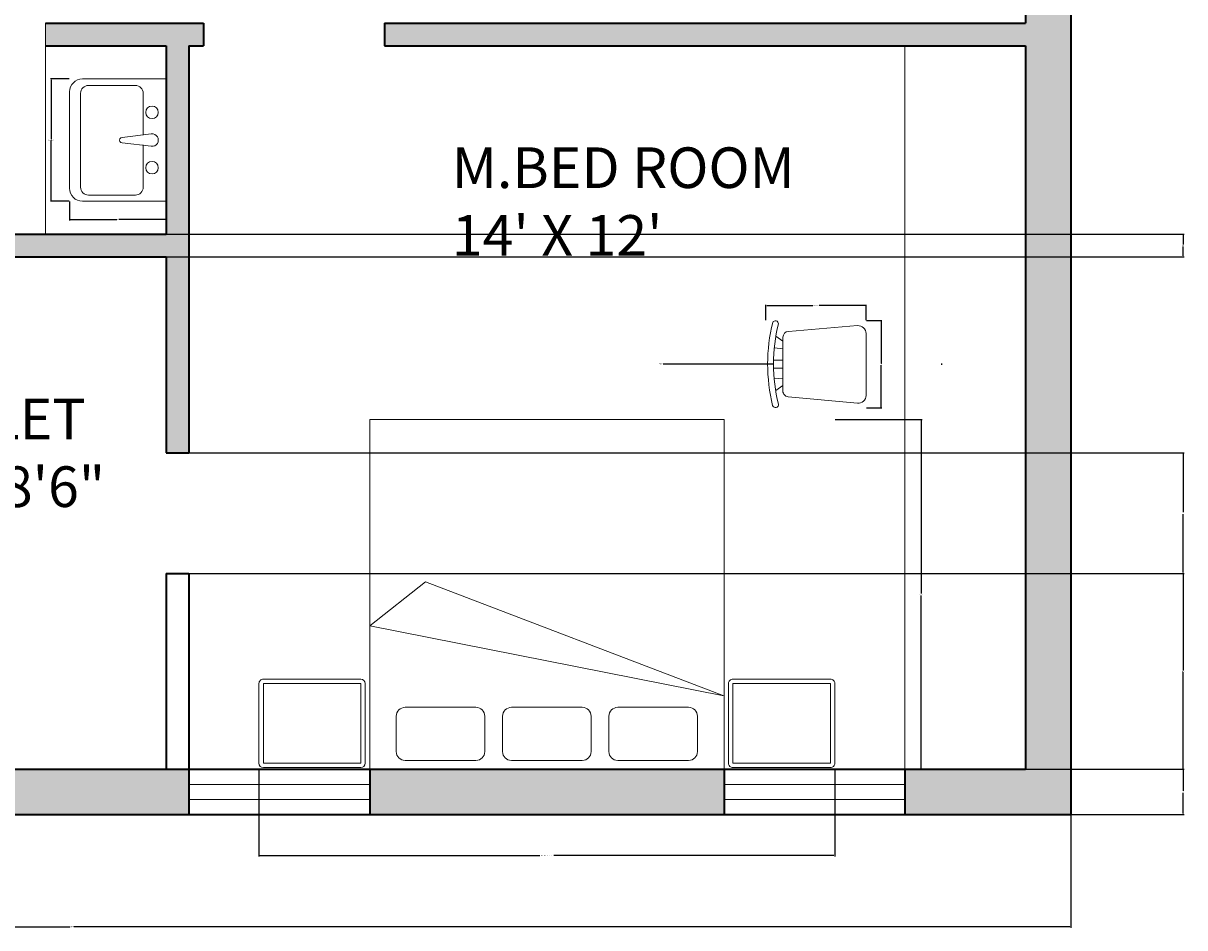
# Model space of a CAD drawing. Units: inches. Extents: x 2 to 2806, y 1095 to 1587.
# Tile 2 of 4: x 2575 to 2806, y 1095 to 1275. Entities that reach past the tile are written whole.
import ezdxf

# ---------------------------------------------------------------- set-up
doc = ezdxf.new("R2010")
doc.units = ezdxf.units.IN
for name, color, linetype, lineweight in [('A-ANNO-DIMS', 2, 'Continuous', 18), ('A-AREA-IDEN', 7, 'Continuous', 25), ('A-FLOR-CASE', 34, 'Continuous', 18), ('A-FLOR-FIXT', 9, 'Continuous', 18), ('A-FURN', 8, 'Continuous', 18), ('A-GLAZ', 4, 'Continuous', 18), ('A-WALL', 7, 'Continuous', 35)]:
    doc.layers.add(name, color=color, linetype=linetype, lineweight=lineweight)
doc.layers.add('A-WALL-PATT', color=18, linetype='Continuous', lineweight=13, true_color=0x000000)
doc.styles.get("Standard").update_dxf_attribs({"font": 'arial.ttf'})
doc.dimstyles.get("Standard").update_dxf_attribs({"dimtxt": 0.18, "dimasz": 0.18, "dimexe": 0.18, "dimexo": 0.0625, "dimgap": 0.09, "dimtad": 0, "dimtih": 1, "dimtoh": 1, "dimdec": 4, "dimzin": 0, "dimdsep": 46, "dimtxsty": 'Standard', "dimcen": 0.09, "dimadec": 0, "dimazin": 0, "dimtfac": 1, "dimtdec": 4, "dimtofl": 0, "dimtmove": 0, "dimatfit": 3, "dimfxl": 1, "dimtolj": 1, "dimtzin": 0, "dimarcsym": 0})

# ---------------------------------------------------------------- blocks, each defined once
blk = doc.blocks.new('A$C34D52403')
for p, q in [((0, 0.4572), (0, 0.061)), ((0.5791, 0.4572), (0, 0.4572)), ((0.5791, 0.061), (0.5791, 0.4572)), ((0.277, 0.2492), (0.2602, 0.387)), ((0.3022, 0.2492), (0.319, 0.387)), ((0.2663, 0.3489), (0.0679, 0.3489)), ((0.5131, 0.3489), (0.3128, 0.3489)), ((0.0308, 0.3118), (0.0308, 0.0892)), ((0.5502, 0.0892), (0.5502, 0.3118)), ((0.0679, 0.0521), (0.5131, 0.0521)), ((0.061, 0), (0.5182, 0))]:
    blk.add_line(p, q)
for centre in [(0.1584, 0.3906), (0.4208, 0.3906)]:
    blk.add_circle(centre, 0.0296)
for centre, radius, start, end in [((0.2896, 0.3906), 0.0296, 353.0422, 186.9578), ((0.0679, 0.3118), 0.0371, 90, 180), ((0.5131, 0.3118), 0.0371, 0, 90), ((0.2896, 0.2491), 0.0125, 179.3528, 0.6472), ((0.061, 0.061), 0.061, 180, 270), ((0.0679, 0.0892), 0.0371, 180, 270), ((0.5131, 0.0892), 0.0371, 270, 0), ((0.5182, 0.061), 0.061, 270, 0)]:
    blk.add_arc(centre, radius, start, end)
blk = doc.blocks.new('A$C793B20D3')
for p, q in [((0.625, 0), (0.625, 1.975)), ((2.625, 1.975), (0.625, 1.975)), ((2.625, 0), (2.625, 1.975)), ((0.575, 1.9405), (0.025, 1.9405)), ((0.025, 1.9405), (0.025, 1.4905)), ((0.575, 1.4905), (0.575, 1.9405)), ((0.825, 1.925), (1.225, 1.925)), ((1.425, 1.925), (1.825, 1.925)), ((2.025, 1.925), (2.425, 1.925)), ((2.65, 1.4905), (2.65, 1.9405)), ((2.675, 1.9655), (3.225, 1.9655)), ((3.25, 1.9405), (3.25, 1.4905)), ((0.775, 1.675), (0.775, 1.875)), ((1.275, 1.675), (1.275, 1.875)), ((1.375, 1.675), (1.375, 1.875)), ((1.875, 1.675), (1.875, 1.875)), ((1.975, 1.675), (1.975, 1.875)), ((2.475, 1.675), (2.475, 1.875)), ((0.825, 1.625), (1.225, 1.625)), ((1.425, 1.625), (1.825, 1.625)), ((2.025, 1.625), (2.425, 1.625)), ((0.6256, 1.5604), (2.3107, 0.9169)), ((0.6256, 1.5604), (2.625, 1.1646)), ((0.025, 1.4905), (0.575, 1.4905)), ((3.225, 1.4655), (2.675, 1.4655)), ((2.3107, 0.9169), (2.625, 1.1646)), ((2.625, 0), (0.625, 0))]:
    blk.add_line(p, q)
at = {"flags": 128}
blk.add_lwpolyline([(0, 1.9405), (0, 1.4905, 0.414214), (0.025, 1.4655), (0.575, 1.4655, 0.414214), (0.6, 1.4905), (0.6, 1.9405, 0.414214), (0.575, 1.9655), (0.025, 1.9655, 0.414214)], format="xyb", close=True, dxfattribs=at)
blk.add_lwpolyline([(3.225, 1.9405), (3.225, 1.4905), (2.675, 1.4905), (2.675, 1.9405)], close=True)
for centre, radius, start, end in [((0.825, 1.875), 0.05, 90, 180), ((1.225, 1.875), 0.05, 0, 90), ((1.425, 1.875), 0.05, 90, 180), ((1.825, 1.875), 0.05, 0, 90), ((2.025, 1.875), 0.05, 90, 180), ((2.425, 1.875), 0.05, 0, 90), ((2.675, 1.9405), 0.025, 90, 180), ((3.225, 1.9405), 0.025, 0, 90), ((0.825, 1.675), 0.05, 180, 270), ((1.225, 1.675), 0.05, 270, 0), ((1.425, 1.675), 0.05, 180, 270), ((1.825, 1.675), 0.05, 270, 0), ((2.025, 1.675), 0.05, 180, 270), ((2.425, 1.675), 0.05, 270, 0), ((2.675, 1.4905), 0.025, 180, 270), ((3.225, 1.4905), 0.025, 270, 0)]:
    blk.add_arc(centre, radius, start, end)
blk = doc.blocks.new('A$C309F5002')
for p, q in [((111.5, 420, 1920), (85.9, 456.6, 1920)), ((355.3, 420, 1920), (91.6, 420, 1920)), ((149.5, 420, 1920), (144.7, 463.9, 1920)), ((199.7, 420, 1920), (199.7, 467, 1920)), ((239.7, 420, 1920), (239.7, 467, 1920)), ((297.4, 420, 1920), (302.1, 463.3, 1920)), ((335.4, 420, 1920), (360.3, 455.6, 1920)), ((54.2, 392.8, 1920), (21.8, 43.7, 1920)), ((414.1, 43.3, 1920), (385.2, 392.5, 1920)), ((61.6, 0, 1920), (374.3, 0, 1920))]:
    blk.add_line(p, q)
for centre, radius, start, end in [((14.6, 457.4, 1920), 15, 105.30285, 282.25466), ((220.1, -382.5, 1920), 879.7, 76.18316, 103.77876), ((423.1, 458.1, 1920), 15.4, 269.91655, 62.44977), ((220.1, -382.5, 1920), 849.7, 76.18316, 103.77876), ((85.3, 389.4, 1920), 31.2, 78.31932, 173.81515), ((355.3, 390, 1920), 30, 4.74462, 90), ((61.6, 40, 1920), 40, 174.69095, 270), ((374.3, 40, 1920), 40, 270, 4.74462)]:
    blk.add_arc(centre, radius, start, end)
blk = doc.blocks.new('WIN-GLAZ-36x9')
for p, q in [((0, 3), (36, 3)), ((0, 0), (36, 0))]:
    blk.add_line(p, q)
blk = doc.blocks.new('*D30')
at = {"layer": 'A-ANNO-DIMS', "color": 0, "lineweight": -2, "transparency": 16777216}
for p, q in [((2621.61, 1126.15), (2621.61, 1108.85)), ((2736.17, 1126.15), (2736.17, 1108.85)), ((2621.79, 1109.03), (2677.51, 1109.03)), ((2735.99, 1109.03), (2680.28, 1109.03))]:
    blk.add_line(p, q, dxfattribs=at)
at = {"layer": 'A-ANNO-DIMS', "color": 0, "transparency": 16777216}
for points in [[(2621.79, 1109.06), (2621.79, 1109), (2621.61, 1109.03)], [(2735.99, 1109.06), (2735.99, 1109), (2736.17, 1109.03)]]:
    blk.add_solid(points, dxfattribs=at)
at = {"layer": 'Defpoints', "color": 0, "transparency": 16777216}
for p in [(2621.61, 1126.21), (2736.17, 1126.21), (2621.61, 1109.03)]:
    blk.add_point(p, dxfattribs=at)
at = {"layer": 'A-ANNO-DIMS', "color": 0, "transparency": 16777216, "insert": (2678.89, 1109.03), "char_height": 0.18, "attachment_point": 5}
blk.add_mtext('\\A1;BED GROUP 115 TYP.', dxfattribs=at)
blk = doc.blocks.new('*D31')
at = {"layer": 'A-ANNO-DIMS', "color": 0, "lineweight": -2, "transparency": 16777216}
for p, q in [((2736.24, 1195.83), (2753.54, 1195.83)), ((2753.36, 1195.65), (2753.36, 1161.2)), ((2753.36, 1126.39), (2753.36, 1160.84)), ((2736.24, 1126.21), (2753.54, 1126.21))]:
    blk.add_line(p, q, dxfattribs=at)
at = {"layer": 'A-ANNO-DIMS', "color": 0, "transparency": 16777216}
for points in [[(2753.33, 1195.65), (2753.39, 1195.65), (2753.36, 1195.83)], [(2753.33, 1126.39), (2753.39, 1126.39), (2753.36, 1126.21)]]:
    blk.add_solid(points, dxfattribs=at)
at = {"layer": 'Defpoints', "color": 0, "transparency": 16777216}
for p in [(2736.17, 1195.83), (2736.17, 1126.21), (2753.36, 1126.21)]:
    blk.add_point(p, dxfattribs=at)
at = {"layer": 'A-ANNO-DIMS', "color": 0, "transparency": 16777216, "insert": (2753.36, 1161.02), "char_height": 0.18, "attachment_point": 5}
blk.add_mtext('\\A1;70 TYP.', dxfattribs=at)
blk = doc.blocks.new('*D46')
at = {"layer": 'A-ANNO-DIMS', "color": 0, "lineweight": -2, "transparency": 16777216}
for p, q in [((2583.87, 1263.63), (2580.11, 1263.63)), ((2580.29, 1263.45), (2580.29, 1251.65)), ((2580.29, 1239.48), (2580.29, 1251.28)), ((2583.87, 1239.3), (2580.11, 1239.3))]:
    blk.add_line(p, q, dxfattribs=at)
at = {"layer": 'A-ANNO-DIMS', "color": 0, "transparency": 16777216}
for points in [[(2580.26, 1263.45), (2580.32, 1263.45), (2580.29, 1263.63)], [(2580.26, 1239.48), (2580.32, 1239.48), (2580.29, 1239.3)]]:
    blk.add_solid(points, dxfattribs=at)
at = {"layer": 'Defpoints', "color": 0, "transparency": 16777216}
for p in [(2583.94, 1263.63), (2580.29, 1239.3), (2583.94, 1239.3)]:
    blk.add_point(p, dxfattribs=at)
at = {"layer": 'A-ANNO-DIMS', "color": 0, "transparency": 16777216, "insert": (2580.29, 1251.46), "char_height": 0.18, "attachment_point": 5}
blk.add_mtext('\\A1;BASIN 24', dxfattribs=at)
blk = doc.blocks.new('*D47')
at = {"layer": 'A-ANNO-DIMS', "color": 0, "lineweight": -2, "transparency": 16777216}
for p, q in [((2583.94, 1239.24), (2583.94, 1235.47)), ((2603.14, 1239.24), (2603.14, 1235.47)), ((2584.12, 1235.65), (2593.33, 1235.65)), ((2602.96, 1235.65), (2593.75, 1235.65))]:
    blk.add_line(p, q, dxfattribs=at)
at = {"layer": 'A-ANNO-DIMS', "color": 0, "transparency": 16777216}
for points in [[(2584.12, 1235.68), (2584.12, 1235.62), (2583.94, 1235.65)], [(2602.96, 1235.68), (2602.96, 1235.62), (2603.14, 1235.65)]]:
    blk.add_solid(points, dxfattribs=at)
at = {"layer": 'Defpoints', "color": 0, "transparency": 16777216}
for p in [(2583.94, 1239.3), (2603.14, 1239.3), (2603.14, 1235.65)]:
    blk.add_point(p, dxfattribs=at)
at = {"layer": 'A-ANNO-DIMS', "color": 0, "transparency": 16777216, "insert": (2593.54, 1235.65), "char_height": 0.18, "attachment_point": 5}
blk.add_mtext('\\A1;19', dxfattribs=at)
blk = doc.blocks.new('*D50')
at = {"layer": 'A-ANNO-DIMS', "color": 0, "lineweight": -2, "transparency": 16777216}
for p, q in [((2722.48, 1215.59), (2722.48, 1218.69)), ((2722.66, 1218.51), (2731.8, 1218.51)), ((2742.21, 1218.51), (2733.08, 1218.51)), ((2742.39, 1215.59), (2742.39, 1218.69))]:
    blk.add_line(p, q, dxfattribs=at)
at = {"layer": 'A-ANNO-DIMS', "color": 0, "transparency": 16777216}
for points in [[(2722.66, 1218.54), (2722.66, 1218.48), (2722.48, 1218.51)], [(2742.21, 1218.54), (2742.21, 1218.48), (2742.39, 1218.51)]]:
    blk.add_solid(points, dxfattribs=at)
at = {"layer": 'Defpoints', "color": 0, "transparency": 16777216}
for p in [(2722.48, 1218.51), (2722.48, 1215.53), (2742.39, 1215.53)]:
    blk.add_point(p, dxfattribs=at)
at = {"layer": 'A-ANNO-DIMS', "color": 0, "transparency": 16777216, "insert": (2732.44, 1218.51), "char_height": 0.18, "attachment_point": 5}
blk.add_mtext('\\A1;CHAIR 20', dxfattribs=at)
blk = doc.blocks.new('*D51')
at = {"layer": 'A-ANNO-DIMS', "color": 0, "lineweight": -2, "transparency": 16777216}
for p, q in [((2742.46, 1215.53), (2745.56, 1215.53)), ((2745.38, 1215.35), (2745.38, 1207.01)), ((2745.38, 1198.32), (2745.38, 1206.65)), ((2742.46, 1198.14), (2745.56, 1198.14))]:
    blk.add_line(p, q, dxfattribs=at)
at = {"layer": 'A-ANNO-DIMS', "color": 0, "transparency": 16777216}
for points in [[(2745.35, 1215.35), (2745.41, 1215.35), (2745.38, 1215.53)], [(2745.35, 1198.32), (2745.41, 1198.32), (2745.38, 1198.14)]]:
    blk.add_solid(points, dxfattribs=at)
at = {"layer": 'Defpoints', "color": 0, "transparency": 16777216}
for p in [(2742.39, 1215.53), (2745.38, 1215.53), (2742.39, 1198.14)]:
    blk.add_point(p, dxfattribs=at)
at = {"layer": 'A-ANNO-DIMS', "color": 0, "transparency": 16777216, "insert": (2745.38, 1206.83), "char_height": 0.18, "attachment_point": 5}
blk.add_mtext('\\A1;17', dxfattribs=at)
blk = doc.blocks.new('*D54')
at = {"layer": 'A-ANNO-DIMS', "color": 0, "lineweight": -2, "transparency": 16777216}
for p, q in [((2385.64, 1117.15), (2385.64, 1094.67)), ((2783.14, 1117.15), (2783.14, 1094.67)), ((2385.82, 1094.85), (2584, 1094.85)), ((2782.96, 1094.85), (2584.79, 1094.85))]:
    blk.add_line(p, q, dxfattribs=at)
at = {"layer": 'A-ANNO-DIMS', "color": 0, "transparency": 16777216}
for points in [[(2385.82, 1094.88), (2385.82, 1094.82), (2385.64, 1094.85)], [(2782.96, 1094.88), (2782.96, 1094.82), (2783.14, 1094.85)]]:
    blk.add_solid(points, dxfattribs=at)
at = {"layer": 'Defpoints', "color": 0, "transparency": 16777216}
for p in [(2385.64, 1117.21), (2783.14, 1117.21), (2783.14, 1094.85)]:
    blk.add_point(p, dxfattribs=at)
at = {"layer": 'A-ANNO-DIMS', "color": 0, "transparency": 16777216, "insert": (2584.39, 1094.85), "char_height": 0.18, "attachment_point": 5}
blk.add_mtext('\\A1;397.5', dxfattribs=at)
blk = doc.blocks.new('*D73')
at = {"layer": 'A-ANNO-DIMS', "color": 0, "lineweight": -2, "transparency": 16777216}
for p, q in [((2607.71, 1126.21), (2805.68, 1126.21)), ((2805.5, 1126.03), (2805.5, 1121.9)), ((2805.5, 1117.39), (2805.5, 1121.53)), ((2607.71, 1117.21), (2805.68, 1117.21))]:
    blk.add_line(p, q, dxfattribs=at)
at = {"layer": 'A-ANNO-DIMS', "color": 0, "transparency": 16777216}
for points in [[(2805.47, 1126.03), (2805.53, 1126.03), (2805.5, 1126.21)], [(2805.47, 1117.39), (2805.53, 1117.39), (2805.5, 1117.21)]]:
    blk.add_solid(points, dxfattribs=at)
at = {"layer": 'Defpoints', "color": 0, "transparency": 16777216}
for p in [(2607.64, 1126.21), (2805.5, 1126.21), (2607.64, 1117.21)]:
    blk.add_point(p, dxfattribs=at)
at = {"layer": 'A-ANNO-DIMS', "color": 0, "transparency": 16777216, "insert": (2805.5, 1121.71), "char_height": 0.18, "attachment_point": 5}
blk.add_mtext('\\A1;9', dxfattribs=at)
blk = doc.blocks.new('*D74')
at = {"layer": 'A-ANNO-DIMS', "color": 0, "lineweight": -2, "transparency": 16777216}
for p, q in [((2607.71, 1165.2), (2805.68, 1165.2)), ((2805.5, 1165.02), (2805.5, 1145.89)), ((2805.5, 1126.39), (2805.5, 1145.52)), ((2607.71, 1126.21), (2805.68, 1126.21))]:
    blk.add_line(p, q, dxfattribs=at)
at = {"layer": 'A-ANNO-DIMS', "color": 0, "transparency": 16777216}
for points in [[(2805.47, 1165.02), (2805.53, 1165.02), (2805.5, 1165.2)], [(2805.47, 1126.39), (2805.53, 1126.39), (2805.5, 1126.21)]]:
    blk.add_solid(points, dxfattribs=at)
at = {"layer": 'Defpoints', "color": 0, "transparency": 16777216}
for p in [(2607.64, 1165.2), (2805.5, 1165.2), (2607.64, 1126.21)]:
    blk.add_point(p, dxfattribs=at)
at = {"layer": 'A-ANNO-DIMS', "color": 0, "transparency": 16777216, "insert": (2805.5, 1145.71), "char_height": 0.18, "attachment_point": 5}
blk.add_mtext('\\A1;38.99', dxfattribs=at)
blk = doc.blocks.new('*D75')
at = {"layer": 'A-ANNO-DIMS', "color": 0, "lineweight": -2, "transparency": 16777216}
for p, q in [((2607.71, 1189.2), (2805.68, 1189.2)), ((2805.5, 1189.02), (2805.5, 1177.38)), ((2805.5, 1165.38), (2805.5, 1177.02)), ((2607.71, 1165.2), (2805.68, 1165.2))]:
    blk.add_line(p, q, dxfattribs=at)
at = {"layer": 'A-ANNO-DIMS', "color": 0, "transparency": 16777216}
for points in [[(2805.47, 1189.02), (2805.53, 1189.02), (2805.5, 1189.2)], [(2805.47, 1165.38), (2805.53, 1165.38), (2805.5, 1165.2)]]:
    blk.add_solid(points, dxfattribs=at)
at = {"layer": 'Defpoints', "color": 0, "transparency": 16777216}
for p in [(2607.64, 1189.2), (2805.5, 1189.2), (2607.64, 1165.2)]:
    blk.add_point(p, dxfattribs=at)
at = {"layer": 'A-ANNO-DIMS', "color": 0, "transparency": 16777216, "insert": (2805.5, 1177.2), "char_height": 0.18, "attachment_point": 5}
blk.add_mtext('\\A1;24', dxfattribs=at)
blk = doc.blocks.new('*D76')
at = {"layer": 'A-ANNO-DIMS', "color": 0, "lineweight": -2, "transparency": 16777216}
for p, q in [((2603.21, 1232.71), (2805.68, 1232.71)), ((2805.5, 1232.53), (2805.5, 1230.64)), ((2805.5, 1228.39), (2805.5, 1230.28)), ((2603.21, 1228.21), (2805.68, 1228.21))]:
    blk.add_line(p, q, dxfattribs=at)
at = {"layer": 'A-ANNO-DIMS', "color": 0, "transparency": 16777216}
for points in [[(2805.47, 1232.53), (2805.53, 1232.53), (2805.5, 1232.71)], [(2805.47, 1228.39), (2805.53, 1228.39), (2805.5, 1228.21)]]:
    blk.add_solid(points, dxfattribs=at)
at = {"layer": 'Defpoints', "color": 0, "transparency": 16777216}
for p in [(2603.14, 1232.71), (2805.5, 1232.71), (2603.14, 1228.21)]:
    blk.add_point(p, dxfattribs=at)
at = {"layer": 'A-ANNO-DIMS', "color": 0, "transparency": 16777216, "insert": (2805.5, 1230.46), "char_height": 0.18, "attachment_point": 5}
blk.add_mtext('\\A1;4.5', dxfattribs=at)
blk = doc.blocks.new('*D77')
at = {"layer": 'A-ANNO-DIMS', "color": 0, "lineweight": -2, "transparency": 16777216}
for p, q in [((2702.04, 1206.9), (2722.64, 1206.89)), ((2757.36, 1206.88), (2757.54, 1206.88)), ((2757.45, 1206.79), (2757.45, 1206.97))]:
    blk.add_line(p, q, dxfattribs=at)
at = {"layer": 'A-ANNO-DIMS', "color": 0, "transparency": 16777216}
blk.add_solid([(2722.64, 1206.92), (2722.64, 1206.86), (2722.82, 1206.89)], dxfattribs=at)
at = {"layer": 'Defpoints', "color": 0, "transparency": 16777216}
for p in [(2722.82, 1206.89), (2757.45, 1206.88)]:
    blk.add_point(p, dxfattribs=at)
at = {"layer": 'A-ANNO-DIMS', "color": 0, "transparency": 16777216, "insert": (2701.56, 1206.9), "char_height": 0.18, "attachment_point": 5}
blk.add_mtext('\\A1;R34.63', dxfattribs=at)
blk = doc.blocks.new('*D78')
at = {"layer": 'A-ANNO-DIMS', "color": 0, "lineweight": -2, "transparency": 16777216}
for p, q in [((2703.93, 1206.9), (2723.82, 1206.89)), ((2757.36, 1206.88), (2757.54, 1206.88)), ((2757.45, 1206.79), (2757.45, 1206.97))]:
    blk.add_line(p, q, dxfattribs=at)
at = {"layer": 'A-ANNO-DIMS', "color": 0, "transparency": 16777216}
blk.add_solid([(2723.82, 1206.92), (2723.82, 1206.86), (2724, 1206.89)], dxfattribs=at)
at = {"layer": 'Defpoints', "color": 0, "transparency": 16777216}
for p in [(2724, 1206.89), (2757.45, 1206.88)]:
    blk.add_point(p, dxfattribs=at)
at = {"layer": 'A-ANNO-DIMS', "color": 0, "transparency": 16777216, "insert": (2703.45, 1206.9), "char_height": 0.18, "attachment_point": 5}
blk.add_mtext('\\A1;R33.45', dxfattribs=at)

msp = doc.modelspace()

# ---------------------------------------------------------------- hatches: boundary and pattern name
at = {"layer": 'A-WALL-PATT'}
h = msp.add_hatch(color=256, dxfattribs=at)
h.dxf.hatch_style = 1
h.paths.add_polyline_path([(2444, 1564.2135), (2385.6427, 1564.2135), (2385.6427, 1465.2135), (2394.6427, 1465.2135), (2394.6427, 1555.2135), (2444, 1555.2135)])
h.paths.add_polyline_path([(2540, 1564.2135), (2480, 1564.2135), (2480, 1555.2135), (2514.6427, 1555.2135), (2514.6427, 1448.7135), (2550.1001, 1448.7135), (2550.1001, 1453.2135), (2519.1427, 1453.2135), (2519.1427, 1555.2135), (2540, 1555.2135)])
h.paths.add_polyline_path([(2619.6427, 1564.2135), (2564, 1564.2135), (2564, 1555.2135), (2579.1427, 1555.2135), (2579.1427, 1453.2135), (2577.7846, 1453.2135), (2577.7846, 1448.7135), (2648.1427, 1448.7135), (2648.1427, 1497.3535), (2643.6427, 1497.3535), (2643.6427, 1453.2135), (2583.6427, 1453.2135), (2583.6427, 1555.2135), (2619.6427, 1555.2135)])
h.paths.add_polyline_path([(2658, 1564.2135), (2643.6427, 1564.2135), (2643.6427, 1555.2135), (2643.6427, 1521.3535), (2648.1427, 1521.3535), (2648.1427, 1555.2135), (2658, 1555.2135)])
h.paths.add_polyline_path([(2783.1427, 1564.2135), (2730, 1564.2135), (2730, 1555.2135), (2774.1427, 1555.2135), (2774.1427, 1465.3633), (2783.1427, 1465.3633)])
h.paths.add_polyline_path([(2783.1427, 1429.3633), (2774.1427, 1429.3633), (2774.1427, 1411.2135), (2610.5887, 1411.2135), (2610.5887, 1406.7135), (2774.1427, 1406.7135), (2774.1427, 1394.7135), (2783.1427, 1394.7135)])
h.paths.add_polyline_path([(2783.1427, 1358.7135), (2774.1427, 1358.7135), (2774.1427, 1336), (2783.1427, 1336)])
h.paths.add_polyline_path([(2783.1427, 1300), (2774.1427, 1300), (2774.1427, 1274.7135), (2646.5887, 1274.7135), (2646.5887, 1270.2135), (2774.1427, 1270.2135), (2774.1427, 1126.2135), (2750.1427, 1126.2135), (2750.1427, 1117.2135), (2783.1427, 1117.2135)])
h.paths.add_polyline_path([(2607.6427, 1126.2135), (2567.1427, 1126.2135), (2567.1427, 1117.2135), (2607.6427, 1117.2135)])
h.paths.add_polyline_path([(2714.1427, 1126.2135), (2643.6427, 1126.2135), (2643.6427, 1117.2135), (2714.1427, 1117.2135)])
h.paths.add_polyline_path([(2607.6427, 1270.2135), (2610.5887, 1270.2135), (2610.5887, 1274.7135), (2579.1427, 1274.7135), (2579.1427, 1270.2135), (2603.1427, 1270.2135), (2603.1427, 1232.7135), (2538.6427, 1232.7135), (2538.6427, 1126.2135), (2543.1427, 1126.2135), (2543.1427, 1228.2135), (2603.1427, 1228.2135), (2603.1427, 1189.2001), (2607.6427, 1189.2001)])
h.paths.add_polyline_path([(2543.1427, 1126.2135), (2514.6427, 1126.2135), (2514.6427, 1117.2135), (2543.1427, 1117.2135)], flags=17)
h.paths.add_polyline_path([(2418.6427, 1126.2135), (2394.6427, 1126.2135), (2394.6427, 1270.2135), (2418.6427, 1270.2135), (2543.1427, 1270.2135), (2543.1427, 1274.7135), (2411.1427, 1274.7135), (2411.1427, 1310), (2402.1427, 1310), (2402.1427, 1274.7135), (2385.6427, 1274.7135), (2385.6427, 1117.2135), (2418.6427, 1117.2135)])
h.paths.add_polyline_path([(2543.1427, 1411.2135), (2394.6427, 1411.2135), (2394.6427, 1429.2135), (2385.6427, 1429.2135), (2385.6427, 1406.7135), (2402.1427, 1406.7135), (2402.1427, 1370), (2411.1427, 1370), (2411.1427, 1406.7135), (2543.1427, 1406.7135)])

# ---------------------------------------------------------------- linework, layer by layer
at = {"layer": 'A-FLOR-CASE'}
for p, q in [((2579.1427, 1274.7135), (2579.1427, 1232.7135)), ((2750.1427, 1270.2135), (2750.1427, 1126.2135))]:
    msp.add_line(p, q, dxfattribs=at)
at = {"layer": 'A-WALL'}
for p, q in [((2774.1427, 1358.7135), (2774.1427, 1274.7135)), ((2783.1427, 1358.7135), (2783.1427, 1117.2135)), ((2579.1427, 1274.7135), (2610.5887, 1274.7135)), ((2610.5887, 1274.7135), (2610.5887, 1270.2135)), ((2646.5887, 1274.7135), (2646.5887, 1270.2135)), ((2646.5887, 1274.7135), (2774.1427, 1274.7135)), ((2579.1427, 1270.2135), (2603.1427, 1270.2135)), ((2603.1427, 1270.2135), (2603.1427, 1232.7135)), ((2607.6427, 1270.2135), (2607.6427, 1189.2001)), ((2607.6427, 1270.2135), (2610.5887, 1270.2135)), ((2646.5887, 1270.2135), (2774.1427, 1270.2135)), ((2774.1427, 1270.2135), (2774.1427, 1126.2135)), ((2538.6427, 1232.7135), (2603.1427, 1232.7135)), ((2543.1427, 1228.2135), (2603.1427, 1228.2135)), ((2603.1427, 1228.2135), (2603.1427, 1189.2001)), ((2603.1427, 1189.2001), (2607.6427, 1189.2001)), ((2603.1427, 1165.2001), (2607.6427, 1165.2001)), ((2603.1427, 1165.2001), (2603.1427, 1126.2135)), ((2607.6427, 1165.2001), (2607.6427, 1126.2135)), ((2394.6427, 1126.2135), (2774.1427, 1126.2135)), ((2607.6427, 1126.2135), (2607.6427, 1117.2135)), ((2643.6427, 1126.2135), (2643.6427, 1117.2135)), ((2714.1427, 1126.2135), (2714.1427, 1117.2135)), ((2750.1427, 1126.2135), (2750.1427, 1117.2135)), ((2385.6427, 1117.2135), (2783.1427, 1117.2135))]:
    msp.add_line(p, q, dxfattribs=at)

# ---------------------------------------------------------------- block references
at = {"layer": 'A-FLOR-FIXT', "xscale": 42.00717080430623, "yscale": 42.00717080430623, "zscale": 42.00717080430623, "rotation": 270}
msp.add_blockref('A$C34D52403', (2583.937, 1263.627), dxfattribs=at)
at = {"layer": 'A-FURN'}
for name, p, xscale, yscale, zscale, rotation in [('A$C309F5002', (2742.3939, 1198.2135), 0.0393700787401575, 0.0393700787401575, 0.0393700787401575, 90), ('A$C793B20D3', (2736.1741, 1195.8324), 35.25, 35.25, 35.25, 180)]:
    msp.add_blockref(name, p, dxfattribs=dict(at, xscale=xscale, yscale=yscale, zscale=zscale, rotation=rotation))
at = {"layer": 'A-GLAZ', "rotation": 180}
msp.add_blockref('WIN-GLAZ-36x9', (2643.6427, 1123.2135), dxfattribs=at)
at = {"layer": 'A-GLAZ'}
msp.add_blockref('WIN-GLAZ-36x9', (2714.1427, 1120.2135), dxfattribs=at)

# ---------------------------------------------------------------- texts
at = {"layer": 'A-AREA-IDEN', "insert": (2660, 1250), "char_height": 8.089392, "width": 85.242088, "attachment_point": 1}
msp.add_mtext("M.BED ROOM \\P14' X 12'", dxfattribs=at)
at = {"layer": 'A-AREA-IDEN', "insert": (2550, 1200), "char_height": 8.08939, "attachment_point": 1}
msp.add_mtext('TOILET\\P5\' X 8\'6"', dxfattribs=at)

# ---------------------------------------------------------------- dimensions: what is measured, and where the dimension line sits
at = {"layer": 'A-ANNO-DIMS'}
for base, p1, p2, angle, text, picture, middle in [((2580.2879, 1239.2999), (2583.937, 1263.627), (2583.937, 1239.2999), 270, 'BASIN <>', '*D46', (2580.2879, 1251.4635)), ((2722.4839, 1218.5136), (2742.3939, 1215.5271), (2722.4839, 1215.5271), 180, 'CHAIR <>', '*D50', (2732.4389, 1218.5136)), ((2753.3583, 1126.2135), (2736.1739, 1195.8322), (2736.1739, 1126.2135), 270, '<> TYP.', '*D31', (2753.3583, 1161.0228)), ((2621.6114, 1109.0291), (2736.1739, 1126.2135), (2621.6114, 1126.2135), 180, 'BED GROUP <> TYP.', '*D30', (2678.8927, 1109.0291))]:
    dim = msp.add_linear_dim(base=base, p1=p1, p2=p2, angle=angle, text=text, dimstyle='Standard', override={"dimdec": 0, "dimlfac": 1, "dimrnd": 0, "dimzin": 0, "dimdsep": 46, "dimlunit": 2}, dxfattribs=at)
    dim.commit()
    dim.dimension.update_dxf_attribs({"geometry": picture, "text_midpoint": middle})
for base, p1, p2, override, picture, middle in [((2603.1427, 1235.6508), (2583.937, 1239.2999), (2603.1427, 1239.2999), {"dimdec": 0, "dimlfac": 1, "dimrnd": 0, "dimzin": 0, "dimdsep": 46, "dimlunit": 2}, '*D47', (2593.5399, 1235.6508)), ((2783.1427, 1094.8535), (2385.6427, 1117.2135), (2783.1427, 1117.2135), {"dimdec": 1, "dimlfac": 1, "dimrnd": 0, "dimzin": 0, "dimdsep": 46, "dimlunit": 2}, '*D54', (2584.3927, 1094.8535))]:
    dim = msp.add_linear_dim(base=base, p1=p1, p2=p2, dimstyle='Standard', override=override, dxfattribs=at)
    dim.commit()
    dim.dimension.update_dxf_attribs({"geometry": picture, "text_midpoint": middle})
for base, p1, p2, override, picture, middle in [((2805.5027, 1232.7135), (2603.1427, 1228.2135), (2603.1427, 1232.7135), {"dimdec": 1, "dimlfac": 1, "dimrnd": 0, "dimzin": 0, "dimdsep": 46, "dimlunit": 2}, '*D76', (2805.5027, 1230.4635)), ((2745.3804, 1215.5271), (2742.3939, 1198.1372), (2742.3939, 1215.5271), {"dimdec": 0, "dimlfac": 1, "dimrnd": 0, "dimzin": 0, "dimdsep": 46, "dimlunit": 2}, '*D51', (2745.3804, 1206.8322)), ((2805.5027, 1189.2001), (2607.6427, 1165.2001), (2607.6427, 1189.2001), {"dimdec": 0, "dimlfac": 1, "dimrnd": 0, "dimzin": 0, "dimdsep": 46, "dimlunit": 2}, '*D75', (2805.5027, 1177.2001)), ((2805.5027, 1165.2001), (2607.6427, 1126.2135), (2607.6427, 1165.2001), {"dimdec": 2, "dimlfac": 1, "dimrnd": 0, "dimzin": 0, "dimdsep": 46, "dimlunit": 2}, '*D74', (2805.5027, 1145.7068)), ((2805.5027, 1126.2135), (2607.6427, 1117.2135), (2607.6427, 1126.2135), {"dimdec": 0, "dimlfac": 1, "dimrnd": 0, "dimzin": 0, "dimdsep": 46, "dimlunit": 2}, '*D73', (2805.5027, 1121.7135))]:
    dim = msp.add_linear_dim(base=base, p1=p1, p2=p2, angle=90, dimstyle='Standard', override=override, dxfattribs=at)
    dim.commit()
    dim.dimension.update_dxf_attribs({"geometry": picture, "text_midpoint": middle})
for mpoint, picture, middle in [((2722.8179, 1206.892), '*D77', (2702.038, 1206.8992)), ((2723.999, 1206.891), '*D78', (2703.9278, 1206.8976))]:
    dim = msp.add_radius_dim(center=(2757.4511, 1206.88), mpoint=mpoint, dimstyle='Standard', override={"dimdec": 2, "dimlfac": 1, "dimrnd": 0, "dimzin": 0, "dimdsep": 46, "dimlunit": 2}, dxfattribs=at)
    dim.commit()
    dim.dimension.update_dxf_attribs({"geometry": picture, "text_midpoint": middle, "dimtype": 164})

doc.saveas('drawing.dxf')
